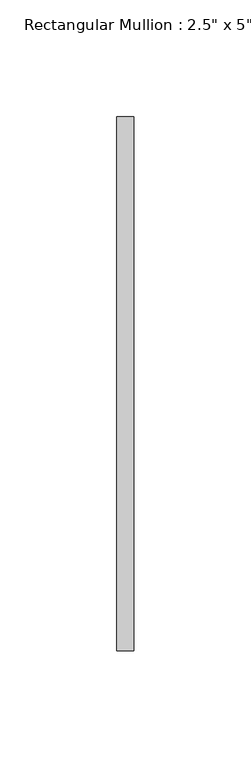
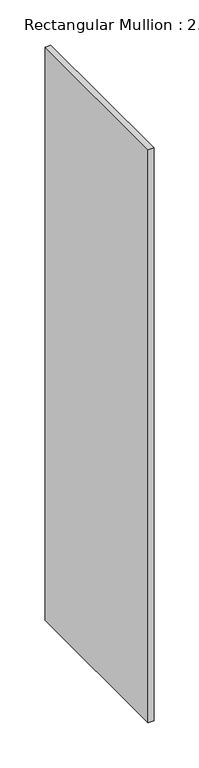
"""IFC4 building model written with IfcOpenShell, lengths in millimetres: member geometry."""

from ifc_helpers import new_model, si_unit, frame, origin, place, context, project, spatial, polyline, outline, extrude, source, transform, mapped, element, save


def member_330b65be(model_context):
    return source(origin(), model_context, "Body", "SweptSolid", [
        extrude(outline(polyline([(0.0, 114.3), (0.0, -114.3), (-7.239, -114.3), (-7.239, 114.3), (0.0, 114.3)])), frame((0.0, 0.0, -774.7), z_axis=(0.0, 0.0, 1.0), x_axis=(1.0, 0.0, 0.0)), (0.0, 0.0, 1.0), 774.7),
    ])


if __name__ == "__main__":
    model = new_model("IFC4")
    model_context = context("Model", 3, world=origin())
    ifc_project = project(units=[si_unit("LENGTHUNIT", "METRE", prefix="MILLI")], contexts=[model_context])
    site = spatial("IfcSite", under=ifc_project)
    building = spatial("IfcBuilding", under=site)
    placement = place(None, origin())
    member_shape = member_330b65be(model_context)
    element("IfcMember", 1, ObjectType="Rectangular Mullion : 2.5\" x 5\" rectangular", at=placement, inside=building, context=model_context, shape_type="MappedRepresentation", body=[
        mapped(member_shape, transform((0.0, 0.0, 0.0), x_axis=(1.0, 0.0, 0.0), y_axis=(0.0, 1.0, 0.0), z_axis=(0.0, 0.0, 1.0))),
    ])
    save(model, "model.ifc")

# Revit data of these elements
# Type "Rectangular Mullion : 2.5\" x 5\" rectangular"
#   built-in parameter 1007304 = 0.75 (stored number, unit not read)
#   built-in parameter 1007301 = 0.011875 (stored number, unit not read)
#   built-in parameter 1007300 = 0.011875 (stored number, unit not read)
# Element 1 (IfcMember, "Rectangular Mullion : 2.5\" x 5\" rectangular")
#   Materials on its faces: "WINDOW GLASS MATERIAL"
# Materials
#   "WINDOW GLASS MATERIAL": class "Generic", colour RGB 120 120 120, transparency 0, Cost = 0
